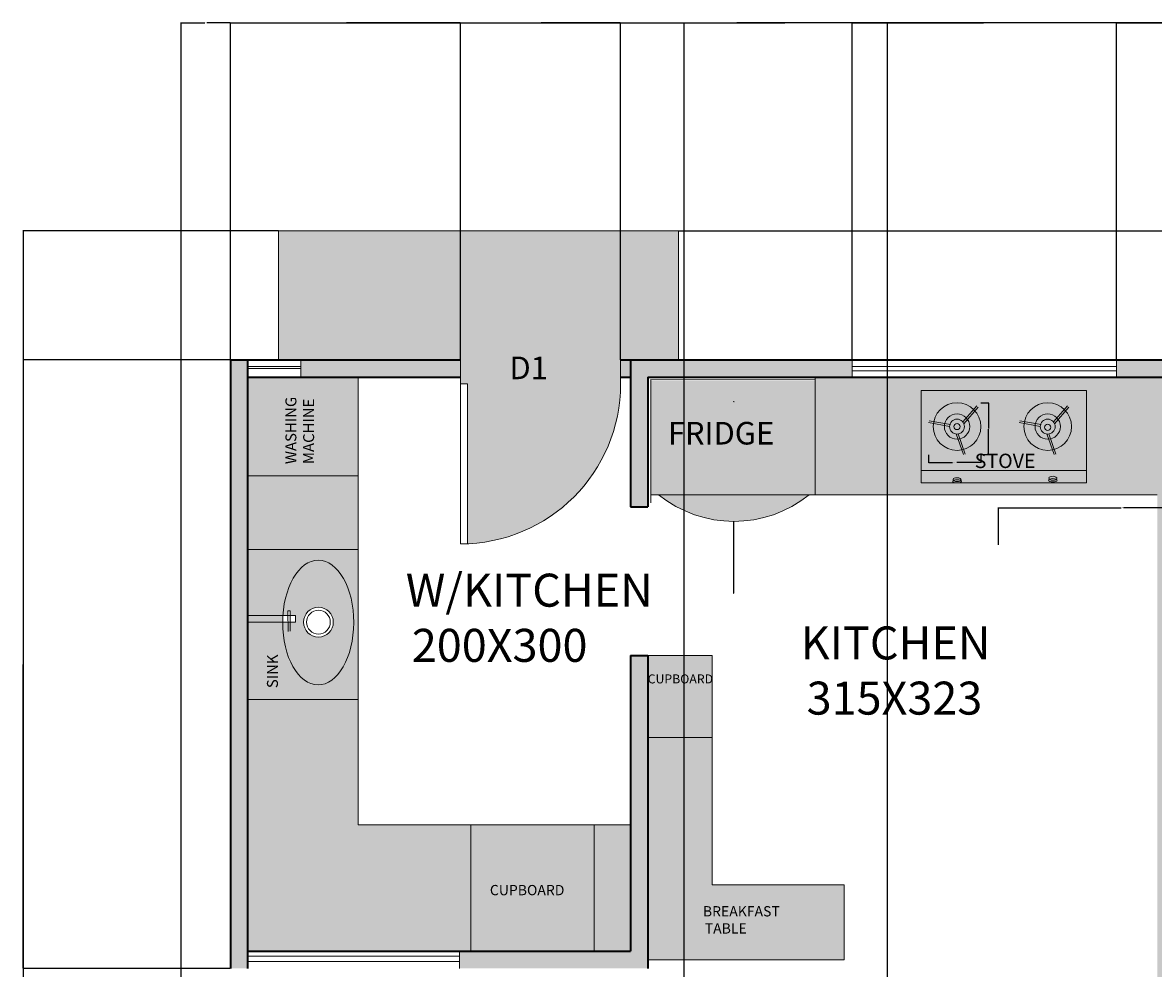
# Model space of a CAD drawing. Units: inches. Extents: x 192 to 1361, y -1362 to 367.
# Tile 19 of 23: x 192 to 783, y -127 to 367. Entities that reach past the tile are written whole.
import ezdxf

# ---------------------------------------------------------------- set-up
doc = ezdxf.new("R2010")
doc.units = ezdxf.units.IN
doc.header["$MEASUREMENT"] = 0
for name, color, linetype, lineweight in [('A-ANNO-DIMS', 2, 'Continuous', 18), ('A-AREA-IDEN', 7, 'Continuous', 18), ('A-DOOR', 4, 'Continuous', 18), ('A-EQPM', 8, 'Continuous', 18), ('A-FLOR-CASE', 32, 'Continuous', 18), ('A-FLOR-FIXT', 8, 'Continuous', 18), ('A-FLOR-STRS', 7, 'Continuous', 18), ('A-WALL-PATT', 250, 'Continuous', 13), ('text', 7, 'Continuous', 18), ('walls', 7, 'Continuous', 35), ('windows', 4, 'Continuous', 18)]:
    doc.layers.add(name, color=color, linetype=linetype, lineweight=lineweight)
for name, color, linetype, lineweight, true_color in [('A-EQPM-PATT', 251, 'Continuous', 13, 0x636466), ('A-FLOR-CASE-PATT', 9, 'Continuous', 13, 0xc7c8ca), ('A-FLOR-FIXT-PATT', 251, 'Continuous', 13, 0x636466), ('A-FLOR-STRS-PATT', 252, 'Continuous', 13, 0x939598)]:
    doc.layers.add(name, color=color, linetype=linetype, lineweight=lineweight, true_color=true_color)
doc.styles.get("Standard").update_dxf_attribs({"font": 'arial.ttf'})
doc.dimstyles.get("Standard").update_dxf_attribs({"dimtxt": 0.18, "dimasz": 0.18, "dimexe": 0.18, "dimexo": 0.0625, "dimgap": 0.09, "dimtad": 0, "dimtih": 1, "dimtoh": 1, "dimzin": 0, "dimdsep": 46, "dimlunit": 3, "dimtxsty": 'Standard', "dimcen": 0.09, "dimadec": 0, "dimazin": 0, "dimtfac": 1, "dimtofl": 0, "dimtmove": 0, "dimatfit": 3, "dimfxl": 1, "dimtolj": 1, "dimtzin": 0, "dimarcsym": 0})

# ---------------------------------------------------------------- blocks, each defined once
blk = doc.blocks.new('*U2')
for p, q in [((0, 0), (-1e-16, -5.999999999999999)), ((40, -6e-16), (40, -6))]:
    blk.add_line(p, q)
blk.add_lwpolyline([(0, 0), (5.6e-15, 40), (1.750000000000007, 40), (1.749999999999998, -7e-16)], close=True)
blk.add_arc((0, 0), 40, 0, 90)
blk = doc.blocks.new('COOKTOP-BURNER')
for p, q in [((2.998043829084622, 2.479431517935921), (10.32791550119827, 10.87990728422207)), ((3.605004346216333, 1.462802486064987), (11.02729633620413, 10.21636973317069)), ((-3.912598951481527, -2.84e-14), (-14.8525602053071, 2.147617193399554)), ((-3.335652644571382, 1.033957743843728), (-14.62761024594374, 3.085067534771468)), ((-0.5356780643953698, -3.853426587660607), (3.333987552905909, -14.65810362865281)), ((0.6482287596465995, -3.836097875688011), (4.258318341358403, -14.38419083685303))]:
    blk.add_line(p, q)
for radius in [12.42722873055866, 6.60613442143804, 3.890481648582393]:
    blk.add_circle((1.137e-13, -2.84e-14), radius)
blk = doc.blocks.new('*D37')
at = {"layer": 'A-ANNO-DIMS', "color": 0, "lineweight": -2, "transparency": 16777216}
for p, q in [((665.3194969474908, 141.5488445880535), (665.3194969474908, 137.3393762476736)), ((665.4994969474907, 137.5193762476736), (677.8694459856831, 137.5193762476736)), ((692.4192858833568, 137.5193762476736), (680.0493368451646, 137.5193762476736)), ((692.5992858833567, 141.5488445880535), (692.5992858833567, 137.3393762476736))]:
    blk.add_line(p, q, dxfattribs=at)
at = {"layer": 'A-ANNO-DIMS', "color": 0, "transparency": 16777216}
for points in [[(665.4994969474907, 137.5493762476736), (665.4994969474907, 137.4893762476736), (665.3194969474908, 137.5193762476736)], [(692.4192858833568, 137.5493762476736), (692.4192858833568, 137.4893762476736), (692.5992858833567, 137.5193762476736)]]:
    blk.add_solid(points, dxfattribs=at)
at = {"layer": 'Defpoints', "color": 0, "transparency": 16777216}
for p in [(665.3194969474908, 141.6113445880535), (692.5992858833567, 141.6113445880535), (692.5992858833567, 137.5193762476736)]:
    blk.add_point(p, dxfattribs=at)
at = {"layer": 'A-ANNO-DIMS', "color": 0, "transparency": 16777216, "insert": (678.9593914154239, 137.5193762476736), "char_height": 0.18, "attachment_point": 5}
blk.add_mtext('\\A1;BURNER 27 TYP.', dxfattribs=at)
blk = doc.blocks.new('*D38')
at = {"layer": 'A-ANNO-DIMS', "color": 0, "lineweight": -2, "transparency": 16777216}
for p, q in [((692.6617858833569, 168.696676947265), (696.871254223737, 168.696676947265)), ((696.6912542237371, 168.5166769472649), (696.6912542237371, 155.3344405084505)), ((696.6912542237371, 141.7913445880535), (696.6912542237371, 154.9735810268679)), ((692.6617858833569, 141.6113445880535), (696.871254223737, 141.6113445880535))]:
    blk.add_line(p, q, dxfattribs=at)
at = {"layer": 'A-ANNO-DIMS', "color": 0, "transparency": 16777216}
for points in [[(696.661254223737, 168.5166769472649), (696.7212542237371, 168.5166769472649), (696.6912542237371, 168.696676947265)], [(696.661254223737, 141.7913445880535), (696.7212542237371, 141.7913445880535), (696.6912542237371, 141.6113445880535)]]:
    blk.add_solid(points, dxfattribs=at)
at = {"layer": 'Defpoints', "color": 0, "transparency": 16777216}
for p in [(692.5992858833569, 168.696676947265), (696.6912542237371, 168.696676947265), (692.5992858833569, 141.6113445880535)]:
    blk.add_point(p, dxfattribs=at)
at = {"layer": 'A-ANNO-DIMS', "color": 0, "transparency": 16777216, "insert": (696.691254223737, 155.154010767659), "char_height": 0.18, "attachment_point": 5}
blk.add_mtext('\\A1;27 TYP.', dxfattribs=at)
blk = doc.blocks.new('*D45')
at = {"layer": 'A-ANNO-DIMS', "color": 0, "lineweight": -2, "transparency": 16777216}
for p, q in [((701.780963977869, 94.4585869856048), (701.780963977869, 113.9793046531113)), ((701.9609639778689, 113.7993046531113), (765.841371209712, 113.7993046531113)), ((830.9557484279125, 113.7993046531113), (767.0753411960693, 113.7993046531113)), ((831.1357484279124, 94.4585869856048), (831.1357484279124, 113.9793046531113))]:
    blk.add_line(p, q, dxfattribs=at)
at = {"layer": 'A-ANNO-DIMS', "color": 0, "transparency": 16777216}
for points in [[(701.9609639778689, 113.8293046531113), (701.9609639778689, 113.7693046531113), (701.780963977869, 113.7993046531113)], [(830.9557484279125, 113.8293046531113), (830.9557484279125, 113.7693046531113), (831.1357484279124, 113.7993046531113)]]:
    blk.add_solid(points, dxfattribs=at)
at = {"layer": 'Defpoints', "color": 0, "transparency": 16777216}
for p in [(701.780963977869, 113.7993046531113), (701.780963977869, 94.3960869856048), (831.1357484279124, 94.3960869856048)]:
    blk.add_point(p, dxfattribs=at)
at = {"layer": 'A-ANNO-DIMS', "color": 0, "transparency": 16777216, "insert": (766.4583562028906, 113.7993046531113), "char_height": 0.18, "attachment_point": 5}
blk.add_mtext('\\A1;SINK 129', dxfattribs=at)
blk = doc.blocks.new('*D48')
at = {"layer": 'A-ANNO-DIMS', "color": 0, "lineweight": -2, "transparency": 16777216}
for p, q in [((325.6332190000001, 258.5285980000001), (192.162545, 258.5285980000001)), ((192.3425450000001, 258.3485980000001), (192.3425450000002, -429.2150894706685)), ((192.3425450000004, -1117.142706), (192.3425450000002, -429.5790185293316)), ((395.2143240000002, -1117.322706), (192.1625450000004, -1117.322706))]:
    blk.add_line(p, q, dxfattribs=at)
at = {"layer": 'A-ANNO-DIMS', "color": 0, "transparency": 16777216}
for points in [[(192.312545, 258.3485980000001), (192.3725450000001, 258.3485980000001), (192.3425450000001, 258.5285980000001)], [(192.3125450000004, -1117.142706), (192.3725450000004, -1117.142706), (192.3425450000004, -1117.322706)]]:
    blk.add_solid(points, dxfattribs=at)
at = {"layer": 'Defpoints', "color": 0, "transparency": 16777216}
for p in [(325.6957190000001, 258.5285980000001), (192.3425450000004, -1117.322706), (395.2768240000002, -1117.322706)]:
    blk.add_point(p, dxfattribs=at)
at = {"layer": 'A-ANNO-DIMS', "color": 0, "transparency": 16777216, "insert": (192.342545, -429.397054), "char_height": 0.18, "attachment_point": 5}
blk.add_mtext('\\A1;1375.9', dxfattribs=at)
blk = doc.blocks.new('*D49')
at = {"layer": 'A-ANNO-DIMS', "color": 0, "lineweight": -2, "transparency": 16777216}
for p, q in [((274.892545, -399.349572), (274.8925450000001, 367.389667)), ((275.072545, 367.209667), (287.2537032892224, 367.209667)), ((300.365189, 367.209667), (288.1840307107777, 367.209667)), ((300.545189, 191.164493), (300.545189, 367.389667))]:
    blk.add_line(p, q, dxfattribs=at)
at = {"layer": 'A-ANNO-DIMS', "color": 0, "transparency": 16777216}
for points in [[(275.072545, 367.239667), (275.072545, 367.179667), (274.8925450000001, 367.209667)], [(300.365189, 367.239667), (300.365189, 367.179667), (300.545189, 367.209667)]]:
    blk.add_solid(points, dxfattribs=at)
at = {"layer": 'Defpoints', "color": 0, "transparency": 16777216}
for p in [(300.545189, 367.209667), (300.545189, 191.101993), (274.892545, -399.412072)]:
    blk.add_point(p, dxfattribs=at)
at = {"layer": 'A-ANNO-DIMS', "color": 0, "transparency": 16777216, "insert": (287.7188670000001, 367.209667), "char_height": 0.18, "attachment_point": 5}
blk.add_mtext('\\A1;25.653', dxfattribs=at)
blk = doc.blocks.new('*D50')
at = {"layer": 'A-ANNO-DIMS', "color": 0, "lineweight": -2, "transparency": 16777216}
for p, q in [((300.545189, 191.164493), (300.545189, 367.389667)), ((300.725189, 367.209667), (571.3556178929057, 367.209667)), ((842.772718, 367.209667), (572.1422891070941, 367.209667)), ((842.952718, 192.111569), (842.952718, 367.389667))]:
    blk.add_line(p, q, dxfattribs=at)
at = {"layer": 'A-ANNO-DIMS', "color": 0, "transparency": 16777216}
for points in [[(300.725189, 367.239667), (300.725189, 367.179667), (300.545189, 367.209667)], [(842.772718, 367.239667), (842.772718, 367.179667), (842.952718, 367.209667)]]:
    blk.add_solid(points, dxfattribs=at)
at = {"layer": 'Defpoints', "color": 0, "transparency": 16777216}
for p in [(842.952718, 367.209667), (300.545189, 191.101993), (842.952718, 192.049069)]:
    blk.add_point(p, dxfattribs=at)
at = {"layer": 'A-ANNO-DIMS', "color": 0, "transparency": 16777216, "insert": (571.7489534999999, 367.209667), "char_height": 0.18, "attachment_point": 5}
blk.add_mtext('\\A1;542.4', dxfattribs=at)
blk = doc.blocks.new('*D53')
at = {"layer": 'A-ANNO-DIMS', "color": 0, "lineweight": -2, "transparency": 16777216}
for p, q in [((534.6874480000002, 258.5285980000001), (1360.413144000001, 258.5285980000002)), ((1360.233144000001, 258.3485980000002), (1360.233144000001, 225.4707366377901)), ((1360.233144000001, 192.2290690000002), (1360.233144000001, 225.1069303622103)), ((843.0152180000003, 192.0490690000001), (1360.413144000001, 192.0490690000002))]:
    blk.add_line(p, q, dxfattribs=at)
at = {"layer": 'A-ANNO-DIMS', "color": 0, "transparency": 16777216}
for points in [[(1360.203144000001, 258.3485980000002), (1360.263144000001, 258.3485980000002), (1360.233144000001, 258.5285980000002)], [(1360.203144000001, 192.2290690000002), (1360.263144000001, 192.2290690000002), (1360.233144000001, 192.0490690000002)]]:
    blk.add_solid(points, dxfattribs=at)
at = {"layer": 'Defpoints', "color": 0, "transparency": 16777216}
for p in [(534.6249480000002, 258.5285980000001), (1360.233144000001, 258.5285980000002), (842.9527180000003, 192.0490690000001)]:
    blk.add_point(p, dxfattribs=at)
at = {"layer": 'A-ANNO-DIMS', "color": 0, "transparency": 16777216, "insert": (1360.233144000001, 225.2888334999997), "char_height": 0.18, "attachment_point": 5}
blk.add_mtext('\\A1;66.48', dxfattribs=at)
blk = doc.blocks.new('*D61')
at = {"layer": 'A-ANNO-DIMS', "color": 0, "lineweight": -2, "transparency": 16777216}
for p, q in [((300.545189, 191.164493), (300.545189, 367.389667)), ((300.725189, 367.209667), (360.215756803547, 367.209667)), ((420.6179889999999, 367.209667), (361.1274211964529, 367.209667)), ((420.7979889999999, 191.164493), (420.7979889999999, 367.389667))]:
    blk.add_line(p, q, dxfattribs=at)
at = {"layer": 'A-ANNO-DIMS', "color": 0, "transparency": 16777216}
for points in [[(300.725189, 367.239667), (300.725189, 367.179667), (300.545189, 367.209667)], [(420.6179889999999, 367.239667), (420.6179889999999, 367.179667), (420.7979889999999, 367.209667)]]:
    blk.add_solid(points, dxfattribs=at)
at = {"layer": 'Defpoints', "color": 0, "transparency": 16777216}
for p in [(420.7979889999999, 367.209667), (300.545189, 191.101993), (420.7979889999999, 191.101993)]:
    blk.add_point(p, dxfattribs=at)
at = {"layer": 'A-ANNO-DIMS', "color": 0, "transparency": 16777216, "insert": (360.671589, 367.209667), "char_height": 0.18, "attachment_point": 5}
blk.add_mtext('\\A1;120.25', dxfattribs=at)
blk = doc.blocks.new('*D62')
at = {"layer": 'A-ANNO-DIMS', "color": 0, "lineweight": -2, "transparency": 16777216}
for p, q in [((420.7979889999999, 191.164493), (420.7979889999999, 367.389667)), ((420.977989, 367.209667), (462.2743081180082, 367.209667)), ((504.218308, 367.209667), (462.9219888819918, 367.209667)), ((504.398308, 191.164493), (504.398308, 367.389667))]:
    blk.add_line(p, q, dxfattribs=at)
at = {"layer": 'A-ANNO-DIMS', "color": 0, "transparency": 16777216}
for points in [[(420.977989, 367.239667), (420.977989, 367.179667), (420.7979889999999, 367.209667)], [(504.218308, 367.239667), (504.218308, 367.179667), (504.398308, 367.209667)]]:
    blk.add_solid(points, dxfattribs=at)
at = {"layer": 'Defpoints', "color": 0, "transparency": 16777216}
for p in [(504.398308, 367.209667), (420.7979889999999, 191.101993), (504.398308, 191.101993)]:
    blk.add_point(p, dxfattribs=at)
at = {"layer": 'A-ANNO-DIMS', "color": 0, "transparency": 16777216, "insert": (462.5981484999999, 367.209667), "char_height": 0.18, "attachment_point": 5}
blk.add_mtext('\\A1;83.6', dxfattribs=at)
blk = doc.blocks.new('*D63')
at = {"layer": 'A-ANNO-DIMS', "color": 0, "lineweight": -2, "transparency": 16777216}
for p, q in [((504.398308, 191.164493), (504.398308, 367.389667)), ((504.5783079999999, 367.209667), (564.6372506357435, 367.209667)), ((625.222196, 367.209667), (565.1632533642565, 367.209667)), ((625.402196, 191.164493), (625.402196, 367.389667))]:
    blk.add_line(p, q, dxfattribs=at)
at = {"layer": 'A-ANNO-DIMS', "color": 0, "transparency": 16777216}
for points in [[(504.5783079999999, 367.239667), (504.5783079999999, 367.179667), (504.398308, 367.209667)], [(625.222196, 367.239667), (625.222196, 367.179667), (625.402196, 367.209667)]]:
    blk.add_solid(points, dxfattribs=at)
at = {"layer": 'Defpoints', "color": 0, "transparency": 16777216}
for p in [(625.402196, 367.209667), (504.398308, 191.101993), (625.402196, 191.101993)]:
    blk.add_point(p, dxfattribs=at)
at = {"layer": 'A-ANNO-DIMS', "color": 0, "transparency": 16777216, "insert": (564.900252, 367.209667), "char_height": 0.18, "attachment_point": 5}
blk.add_mtext('\\A1;121', dxfattribs=at)
blk = doc.blocks.new('*D64')
at = {"layer": 'A-ANNO-DIMS', "color": 0, "lineweight": -2, "transparency": 16777216}
for p, q in [((625.402196, 191.164493), (625.402196, 367.389667)), ((625.582196, 367.209667), (693.9681959597544, 367.209667)), ((763.2637729999999, 367.209667), (694.8777730402455, 367.209667)), ((763.443773, 191.164493), (763.443773, 367.389667))]:
    blk.add_line(p, q, dxfattribs=at)
at = {"layer": 'A-ANNO-DIMS', "color": 0, "transparency": 16777216}
for points in [[(625.582196, 367.239667), (625.582196, 367.179667), (625.402196, 367.209667)], [(763.2637729999999, 367.239667), (763.2637729999999, 367.179667), (763.443773, 367.209667)]]:
    blk.add_solid(points, dxfattribs=at)
at = {"layer": 'Defpoints', "color": 0, "transparency": 16777216}
for p in [(763.443773, 367.209667), (625.402196, 191.101993), (763.443773, 191.101993)]:
    blk.add_point(p, dxfattribs=at)
at = {"layer": 'A-ANNO-DIMS', "color": 0, "transparency": 16777216, "insert": (694.4229844999999, 367.209667), "char_height": 0.18, "attachment_point": 5}
blk.add_mtext('\\A1;138.04', dxfattribs=at)
blk = doc.blocks.new('*D65')
at = {"layer": 'A-ANNO-DIMS', "color": 0, "lineweight": -2, "transparency": 16777216}
for p, q in [((763.443773, 191.164493), (763.443773, 367.389667)), ((763.6237729999999, 367.209667), (802.6888125143246, 367.209667)), ((842.365189, 367.209667), (803.3001494856751, 367.209667)), ((842.545189, 191.164493), (842.545189, 367.389667))]:
    blk.add_line(p, q, dxfattribs=at)
at = {"layer": 'A-ANNO-DIMS', "color": 0, "transparency": 16777216}
for points in [[(763.6237729999999, 367.239667), (763.6237729999999, 367.179667), (763.443773, 367.209667)], [(842.365189, 367.239667), (842.365189, 367.179667), (842.545189, 367.209667)]]:
    blk.add_solid(points, dxfattribs=at)
at = {"layer": 'Defpoints', "color": 0, "transparency": 16777216}
for p in [(842.545189, 367.209667), (763.443773, 191.101993), (842.545189, 191.101993)]:
    blk.add_point(p, dxfattribs=at)
at = {"layer": 'A-ANNO-DIMS', "color": 0, "transparency": 16777216, "insert": (802.994481, 367.209667), "char_height": 0.18, "attachment_point": 5}
blk.add_mtext('\\A1;79.1', dxfattribs=at)
blk = doc.blocks.new('*D66')
at = {"layer": 'A-ANNO-DIMS', "color": 0, "lineweight": -2, "transparency": 16777216}
for p, q in [((300.4826890000001, 191.101993), (192.1625450000002, 191.101993)), ((192.3425450000002, 190.921993), (192.3425450000002, 32.28395752933149)), ((192.3425450000002, -126.7180070000001), (192.3425450000002, 31.92002847066847)), ((300.4826890000001, -126.898007), (192.1625450000002, -126.8980070000001))]:
    blk.add_line(p, q, dxfattribs=at)
at = {"layer": 'A-ANNO-DIMS', "color": 0, "transparency": 16777216}
for points in [[(192.3125450000002, 190.921993), (192.3725450000002, 190.921993), (192.3425450000002, 191.101993)], [(192.3125450000002, -126.7180070000001), (192.3725450000002, -126.7180070000001), (192.3425450000002, -126.8980070000001)]]:
    blk.add_solid(points, dxfattribs=at)
at = {"layer": 'Defpoints', "color": 0, "transparency": 16777216}
for p in [(300.5451890000001, 191.101993), (192.3425450000002, -126.8980070000001), (300.5451890000001, -126.898007)]:
    blk.add_point(p, dxfattribs=at)
at = {"layer": 'A-ANNO-DIMS', "color": 0, "transparency": 16777216, "insert": (192.3425450000002, 32.10199299999992), "char_height": 0.18, "attachment_point": 5}
blk.add_mtext('\\A1;318', dxfattribs=at)
blk = doc.blocks.new('*D70')
at = {"layer": 'A-ANNO-DIMS', "color": 0, "lineweight": -2, "transparency": 16777216}
for p, q in [((537.571706, -441.835507), (537.571706, 367.389667)), ((537.7517059999998, 367.209667), (590.2778894836289, 367.209667)), ((643.712545, 367.209667), (591.1863615163709, 367.209667)), ((643.892545, -441.835507), (643.892545, 367.389667))]:
    blk.add_line(p, q, dxfattribs=at)
at = {"layer": 'A-ANNO-DIMS', "color": 0, "transparency": 16777216}
for points in [[(537.7517059999998, 367.239667), (537.7517059999998, 367.179667), (537.571706, 367.209667)], [(643.712545, 367.239667), (643.712545, 367.179667), (643.892545, 367.209667)]]:
    blk.add_solid(points, dxfattribs=at)
at = {"layer": 'Defpoints', "color": 0, "transparency": 16777216}
for p in [(643.892545, 367.209667), (537.571706, -441.8980069999999), (643.892545, -441.8980069999999)]:
    blk.add_point(p, dxfattribs=at)
at = {"layer": 'A-ANNO-DIMS', "color": 0, "transparency": 16777216, "insert": (590.7321254999999, 367.209667), "char_height": 0.18, "attachment_point": 5}
blk.add_mtext('\\A1;106.32', dxfattribs=at)
blk = doc.blocks.new('*D73')
at = {"layer": 'A-ANNO-DIMS', "color": 0, "lineweight": -2, "transparency": 16777216}
for p, q in [((563.5042099999997, 169.3224309999999), (563.6842099999996, 169.3224309999999)), ((563.5942099999996, 169.2324309999999), (563.5942099999996, 169.4124309999999)), ((563.5938739999978, 69.15581280021131), (563.5939993962058, 106.538295000001)), ((563.4138739999979, 69.1558128002113), (563.5938739999978, 69.15581280021131))]:
    blk.add_line(p, q, dxfattribs=at)
at = {"layer": 'A-ANNO-DIMS', "color": 0, "transparency": 16777216}
blk.add_solid([(563.5639993962061, 106.5382951006333), (563.6239993962057, 106.5382948993686), (563.5939999999997, 106.7182949999999)], dxfattribs=at)
at = {"layer": 'Defpoints', "color": 0, "transparency": 16777216}
for p in [(563.5942099999997, 169.3224309999999), (563.5939999999997, 106.7182949999999)]:
    blk.add_point(p, dxfattribs=at)
at = {"layer": 'A-ANNO-DIMS', "color": 0, "transparency": 16777216, "insert": (563.0040240682107, 69.15581280021142), "char_height": 0.18, "attachment_point": 5}
blk.add_mtext('\\A1;R62.6', dxfattribs=at)

msp = doc.modelspace()

# ---------------------------------------------------------------- hatches: boundary and pattern name
at = {"layer": 'A-EQPM-PATT'}
h = msp.add_hatch(color=256, dxfattribs=at)
h.dxf.hatch_style = 1
h.paths.add_polyline_path([(520.1272786621957, 180.37523831581), (520.1272786621957, 120.6542820654139), (606.0055655280232, 120.6542820654139), (606.0055655280232, 180.37523831581)])
h.paths.add_polyline_path([(524.2154194657116, 120.6542820654139, 0.3538957662438658), (602.9730012785246, 120.6542820654139)])
h = msp.add_hatch(color=256, dxfattribs=at)
h.dxf.hatch_style = 1
h.paths.add_polyline_path([(654.6941349520653, 133.2965860047039, 0.4472035247863919), (664.4676486712701, 125.6924393581307), (747.8111784828459, 125.6924393581307, 0.3244181347622925), (755.5844684036286, 130.1594570450853), (755.5844684036286, 176.3328940198642, 0.3295456964687013), (747.8111785084185, 181.0248198872323), (661.4957202282897, 181.0248198853133, 0.2614299454499895), (654.6941349520653, 176.569079923764)])
h.paths.add_polyline_path([(667.7448284222395, 156.2694482167063, -1), (692.5992858833569, 156.2694482167063, -1)], flags=16)
h.paths.add_polyline_path([(673.56592273136, 156.2694482167063, -1), (686.778191574236, 156.2694482167063, -1)], flags=0)
h.paths.add_polyline_path([(676.2815755042159, 156.2694482167063, -1), (684.0625388013804, 156.2694482167063, -1)], flags=0)
edge = h.paths.add_edge_path(flags=16)
edge.add_ellipse((680.1596553194548, 127.6653223792632), major_axis=(-2.265511773118937, 0.0641621067748367), ratio=0.3769733725084229, start_angle=41.86570148013669, end_angle=148.3082686719917, ccw=False)
edge.add_ellipse((680.1596553194548, 127.6653223792632), major_axis=(-2.265511773118937, 0.0641621067748367), ratio=0.3769733725084229, start_angle=346.4338229157989, end_angle=401.8657014801367, ccw=False)
edge.add_ellipse((680.1838427235941, 128.5193599934903), major_axis=(-2.108826373640958, 0.136184926067124), ratio=0.4928397098496223, start_angle=169.7196154411588, end_angle=373.72857998463945, ccw=False)
edge.add_ellipse((680.1596553194548, 127.6653223792632), major_axis=(-2.265511773118937, 0.0641621067748367), ratio=0.3769733725084229, start_angle=148.3082686719917, end_angle=192.1304824464878, ccw=False)
h.paths.add_polyline_path([(715.1179190683129, 156.2694482167063, -1), (739.9723765294304, 156.2694482167063, -1)], flags=16)
h.paths.add_polyline_path([(734.1512822203096, 156.2694482167063, -1), (720.9390133774338, 156.2694482167063, -1)], flags=0)
h.paths.add_polyline_path([(731.4356294474538, 156.2694482167063, -1), (723.6546661502894, 156.2694482167063, -1)], flags=0)
h.paths.add_polyline_path([(678.5618801005874, 156.2694482167063, -1), (681.7822342050089, 156.2694482167063, -1)], flags=0)
h.paths.add_polyline_path([(725.934970746661, 156.2694482167063, -1), (729.1553248510824, 156.2694482167063, -1)], flags=0)
edge = h.paths.add_edge_path(flags=16)
edge.add_ellipse((730.2790187730303, 129.2411328864045), major_axis=(-2.108826373640957, 0.1361849260671237), ratio=0.4928397098496223, start_angle=165.0804609789027, end_angle=377.6699463424078, ccw=False)
edge.add_ellipse((730.2119014335817, 128.2018195082961), major_axis=(-2.265511773118937, 0.0641621067748368), ratio=0.3769733725084229, start_angle=342.9101370313131, end_angle=554.300550688774, ccw=False)
at = {"layer": 'A-FLOR-CASE-PATT'}
h = msp.add_hatch(color=256, dxfattribs=at)
h.dxf.hatch_style = 1
h.paths.add_polyline_path([(367.2563921661531, 182.101992675173), (309.5451889353615, 182.101992675173), (309.5451889353615, 130.5475761196903), (367.2563921661531, 130.5475761196903)])
h.paths.add_polyline_path([(367.2563921661531, 13.5566443611624), (309.5451889353615, 13.55664436116237), (309.5451889353615, -117.8980073248269), (426.1374151077765, -117.8980073248269), (426.1374151077765, -51.88342877959076), (367.2563921661531, -51.88342877959076)])
h.paths.add_polyline_path([(367.2563921661531, 130.5475761196903), (309.5451889353615, 130.5475761196903), (309.5451889353615, 91.98957794753846), (367.2563921661531, 91.98957794753848)])
h.paths.add_polyline_path([(490.5683664073912, -51.88342877959076), (426.1374151077765, -51.88342877959079), (426.1374151077765, -117.8980073248269), (490.5683664073913, -117.8980073248269)])
h.paths.add_polyline_path([(509.5451889353614, -51.88342877959076), (490.5683664073912, -51.88342877959076), (490.5683664073913, -117.8980073248269), (509.5451889353614, -117.8980073248269)])
h.paths.add_polyline_path([(552.3161055696219, -6.213326217646681), (518.5451889353614, -6.213326217646681), (518.5451889353614, -122.3395355970042), (621.252934446602, -122.3395355970042), (621.252934446602, -83.2276039636199), (552.3161055696219, -83.22760396361988)])
h.paths.add_polyline_path([(552.3161055696219, 36.60199267517304), (518.5451889353614, 36.60199267517304), (518.5451889353614, -6.213326217646681), (552.3161055696219, -6.213326217646653)])
h = msp.add_hatch(color=256, dxfattribs=at)
h.dxf.hatch_style = 1
h.paths.add_polyline_path([(833.5451889353615, 182.101992675173), (606.035314480534, 182.101992675173), (606.0320695517825, 180.6287964589344), (606.109309992806, 180.6286263256385), (606.0055655280232, 120.6542820654139), (784.8041419739257, 120.6542820658329), (784.8041419739257, -60.49958728474123), (833.5451889353615, -60.49958728474118)])
at = {"layer": 'A-FLOR-FIXT-PATT'}
h = msp.add_hatch(color=256, dxfattribs=at)
h.dxf.hatch_style = 1
edge = h.paths.add_edge_path()
edge.add_ellipse((346.4015860498506, 53.86014095233496), major_axis=(0.0897725345072745, 32.61993048690351), ratio=0.568990406928987, start_angle=89.77278696833508, end_angle=78.68100194365468, ccw=False)
edge.add_line((327.8414083400814, 53.98482425088332), (309.5451889353615, 53.98482425088332))
edge.add_line((309.5451889353615, 53.98482425088332), (309.5451889353615, 13.5566443611624))
edge.add_line((309.5451889353615, 13.5566443611624), (367.2563921661531, 13.5566443611624))
edge.add_line((367.2563921661531, 13.5566443611624), (367.2563921661531, 91.98957794753846))
edge.add_line((367.2563921661531, 91.98957794753848), (309.5451889353615, 91.98957794753846))
edge.add_line((309.5451889353615, 91.98957794753846), (309.5451889353615, 57.60216911136854))
edge.add_line((309.5451889353615, 57.60216911136854), (327.9705352807811, 57.60216911136854))
edge = h.paths.add_edge_path(flags=17)
edge.add_ellipse((346.4015860498506, 53.86014095233496), major_axis=(0.0897725345072745, 32.61993048690351), ratio=0.568990406928987, start_angle=-270.227213031665, end_angle=78.68100194365473)
edge.add_line((327.9705352807811, 57.60216911136854), (330.5969786775669, 57.60216911136854))
edge.add_line((330.5969786775669, 57.60216911136854), (330.5859614346086, 59.90799801485451))
edge.add_line((330.5859614346086, 59.90799801485451), (331.7591235928912, 59.91360337980977))
edge.add_line((331.7591235928912, 59.91360337980977), (331.7701676182649, 57.60216911136854))
edge.add_line((331.7701676182649, 57.60216911136854), (334.4929653930154, 57.60216911136854))
edge.add_line((334.4929653930154, 57.60216911136854), (334.5102490549264, 53.98482425088332))
edge.add_line((334.5102490549264, 53.98482425088332), (327.8414083400814, 53.98482425088332))
h.paths.add_polyline_path([(338.7613475983098, 54.04226685662357, -1), (354.3037905554878, 54.04226685662357, -1)], flags=16)
h.paths.add_polyline_path([(340.3275509583993, 54.04226685662357, -1), (352.7375871953983, 54.04226685662357, -1)], flags=0)
h.paths.add_polyline_path([(352.7375871953983, 54.04226685662357, 1), (340.3275509583993, 54.04226685662357, 1)], flags=0)
edge = h.paths.add_edge_path(flags=17)
edge.add_ellipse((346.4015860498506, 53.86014095233496), major_axis=(0.0897725345072745, 32.61993048690351), ratio=0.568990406928987, start_angle=78.68100194365468, end_angle=89.77278696833503, ccw=False)
edge.add_line((327.9705352807811, 57.60216911136854), (309.5451889353615, 57.60216911136854))
edge.add_line((309.5451889353615, 57.60216911136854), (309.5451889353615, 53.98482425088332))
edge.add_line((309.5451889353615, 53.98482425088332), (327.8414083400814, 53.98482425088332))
at = {"layer": 'A-FLOR-STRS-PATT'}
h = msp.add_hatch(color=256, dxfattribs=at)
h.dxf.hatch_style = 1
h.paths.add_polyline_path([(534.6249481233752, 258.5285978964557), (325.6957187905937, 258.5285978964557), (325.6957187905937, 191.101992675173), (420.7979888647932, 191.101992675173), (420.7979888647932, 178.5619448757428), (424.4555028062937, 178.5619448757428), (424.4555028062937, 95.0416726521634, 0.4014527144963572), (504.3983075276613, 178.5619448757428), (504.3983075276613, 191.101992675173), (534.6249481233752, 191.101992675173)])
at = {"layer": 'A-WALL-PATT'}
h = msp.add_hatch(color=256, dxfattribs=at)
h.dxf.hatch_style = 1
h.paths.add_polyline_path([(309.5451889353615, 191.101992675173), (300.5451889353615, 191.101992675173), (300.5451889353615, -126.898007324827), (309.5451889353615, -126.8980073248269), (309.5451889353615, -117.8980073248269)])
h.paths.add_polyline_path([(420.7979888647932, 191.101992675173), (337.3228677063344, 191.101992675173), (337.3228677063344, 182.101992675173), (420.7979888647932, 182.101992675173)])
h.paths.add_polyline_path([(518.5451889353614, 182.101992675173), (625.402196435898, 182.101992675173), (625.402196435898, 191.101992675173), (509.5451889353614, 191.101992675173), (509.5451889353614, 114.3261562634452), (518.5451889353614, 114.3261562634452)])
h.paths.add_polyline_path([(842.5451889353615, 191.101992675173), (763.4437725118987, 191.101992675173), (763.4437725118989, 182.101992675173), (833.5451889353615, 182.101992675173), (833.5451889353614, 161.1615418579658), (836.8088208065492, 161.1615418579658), (842.5451889353615, 161.1615418579658)])
h.paths.add_polyline_path([(842.5451889353615, -16.5674928553999), (833.5451889353614, -16.56749285539987), (833.5451889353614, -60.49958728474121), (784.8041419739257, -60.49958728474123), (784.8041419739257, -354.6796217638267), (793.8041419739257, -354.6796217638266), (793.8041419739257, -69.49958728474121), (1094.125155398258, -69.49958728474121), (1094.125155398258, -60.49958728474121), (842.5451889353615, -60.49958728474121)])
h.paths.add_polyline_path([(518.5451889353614, 36.60199267517305), (509.5451889353614, 36.60199267517304), (509.5451889353614, -117.8980073248269), (420.2204344382116, -117.8980073248269), (420.2204344382116, -126.898007324827), (518.5451889353614, -126.898007324827)])
h.paths.add_polyline_path([(474.8041419739258, -377.0384258897093), (465.8041419739257, -377.0384258897092), (465.8041419739257, -381.5384258897093), (465.8041419739257, -450.8980073248269), (537.5717061213309, -450.8980073248269), (537.5717061213307, -441.8980073248268), (474.8041419739258, -441.8980073248268)])
h.paths.add_polyline_path([(1162.804141973925, -380.6762896854179), (1204.300070955153, -380.676289685418), (1204.300070955153, -375.6762896854179), (1195.147073967669, -375.6762896854179), (1153.804141973926, -375.6762896854179), (1153.804141973926, -448.4995872847412), (856.5690753709177, -448.4995872847412), (856.5690753709177, -457.499587284741), (1162.804141973925, -457.4995872847412)])
h.paths.add_polyline_path([(1162.804141973925, -525.128007319321), (1153.804141973926, -525.128007319321), (1153.804141973926, -597.4995872847411), (1162.804141973925, -597.4995872847408)], flags=17)
h.paths.add_polyline_path([(1162.804141973925, -60.49958728474121), (1153.804141973926, -60.49958728474121), (1153.804141973926, -69.49958728474121), (1153.804141973926, -177.4732950264469), (1205.888928875302, -177.4732950264469), (1205.888928875302, -172.4732950264469), (1162.804141973925, -172.473295026447)])
h.paths.add_polyline_path([(980.5798651633768, -525.6860130712009), (971.5798651633768, -525.6860130712007), (971.5798651633768, -597.4995872847411), (980.5798651633768, -597.4995872847411)], flags=17)
h.paths.add_polyline_path([(856.5690753709177, -448.4995872847413), (798.7541670773728, -448.4995872847413), (784.8041419739257, -448.4995872847413), (784.8041419739257, -457.4995872847413), (847.5690753709177, -457.4995872847412), (847.5690753709177, -597.4995872847411), (784.8041419739257, -597.4995872847411), (784.8041419739257, -606.4995872847411), (1273.565765398564, -606.4995872847411), (1273.565765398564, -597.4995872847411), (856.5690753709177, -597.4995872847411)])
h.paths.add_polyline_path([(1273.565765398564, -773.8919522895034), (1099.836601134898, -773.8919522895034), (1099.836601134898, -851.9361992714873), (1108.836601134898, -851.9361992714873), (1108.836601134898, -782.8919522895034), (1273.565765398564, -782.8919522895034)])
h.paths.add_polyline_path([(1108.836601134898, -982.9213770098904), (1099.836601134898, -982.9213770098906), (1099.836601134898, -1067.624587332624), (1037.756291549154, -1067.624587332624), (1037.756291549154, -1076.624587332624), (1108.836601134898, -1076.624587332624)])
h.paths.add_polyline_path([(835.0779955891157, -1067.624587332624), (758.8457689766901, -1067.624587332624), (758.8457689766902, -940.2324367059535), (749.8457689766901, -940.2324367059538), (749.8457689766901, -963.1720045953997), (749.8457689766901, -970.4644011765903), (749.8457689766901, -1076.624587332624), (835.0779955891157, -1076.624587332624)])
h.paths.add_polyline_path([(450.3070229383964, -1066.98378940351), (441.3070229383965, -1066.98378940351), (441.3070229383965, -1076.624587332624), (450.3070229383965, -1076.624587332624)])
h.paths.add_polyline_path([(492.8925450663919, -756.4414928502347), (274.8925450663919, -756.4414928502347), (274.8925450663919, -765.4414928502347), (492.8925450663919, -765.4414928502347)])
h.paths.add_polyline_path([(283.8925450663919, -835.2244016542135), (274.8925450663919, -835.2244016542135), (274.8925450663919, -914.4414928502346), (492.8925450663919, -914.4414928502346), (492.8925450663919, -839.9414928502348), (483.8925450663918, -839.9414928502345), (483.8925450663918, -905.4414928502346), (283.8925450663919, -905.4414928502346)])
h.paths.add_polyline_path([(283.8925450663919, -441.898007324827), (283.8925450663918, -375.4296017141059), (281.6021282613037, -375.429601714106), (281.6021282613036, -399.4120715247955), (274.8925450663919, -399.4120715247954), (274.8925450663919, -441.898007324827), (274.8925450663919, -684.5088577166042), (283.8925450663919, -684.5088577166042)])
h = msp.add_hatch(color=256, dxfattribs=at)
h.dxf.hatch_style = 1
h.paths.add_polyline_path([(652.8925450663919, -441.898007324827), (643.8925450663918, -441.898007324827), (643.8925450663918, -457.846133166586), (643.8925450663918, -564.1669721116469), (643.8925450663918, -905.4414928502346), (578.0244629257031, -905.4414928502346), (578.0244629257031, -914.4414928502346), (643.8925450663918, -914.4414928502346), (643.8925450663918, -969.5483657063114), (652.6138145608154, -969.5483657063114), (652.6138145608154, -963.1720045953997), (652.6138145608154, -914.5560273874624)])
h.paths.add_polyline_path([(509.5451889353614, 191.101992675173), (504.3983075276613, 191.1019926751729), (504.3983075276613, 182.1019926751729), (509.5451889353614, 182.1019926751731)])

# ---------------------------------------------------------------- linework, layer by layer
at = {"layer": 'A-EQPM'}
for p, q in [((520.1272786621957, 120.6542820654139), (520.1272786621957, 180.8180142445744)), ((520.1272786621957, 180.8180142445744), (606.109309992806, 180.6286263256385)), ((606.109309992806, 180.6286263256385), (606.0055655280232, 120.6542820654139)), ((661.4957202312175, 175.0385616355948), (661.4957202312175, 126.9029761155034)), ((747.8111785069199, 175.0385616355948), (661.4957202312175, 175.0385616355948)), ((747.8111785069195, 126.9029761155034), (747.8111785069199, 175.0385616355948)), ((520.1272786621957, 116.3888405289696), (520.1272786621957, 161.1454192932534)), ((661.4957202312175, 133.2965860174828), (747.8111785069199, 133.2965860174828)), ((747.8111785069195, 126.9029761155034), (661.4957202312175, 126.9029761155034)), ((606.0055655280232, 120.6542820654139), (520.1272786621957, 120.6542820654139)), ((606.0055655280232, 120.6542820654139), (602.9730012785151, 120.6542820654068))]:
    msp.add_line(p, q, dxfattribs=at)
for centre in [(680.1720571527981, 156.2694482167063), (727.5595086581566, 155.904968577457)]:
    msp.add_circle(centre, 1.610177052210564, dxfattribs=at)
msp.add_arc((563.5942103721195, 169.3224313615276), 62.60413667769229, 231.0226883866979, 308.9773116133019, dxfattribs=at)
for centre, major_axis, ratio in [((730.2790187730303, 129.2411328864045), (-2.108826373640957, 0.1361849260671237), 0.4928397098496223), ((680.1596553194548, 127.6653223792632), (-2.265511773118937, 0.0641621067748367), 0.3769733725084229), ((680.1838427235941, 128.5193599934903), (-2.108826373640957, 0.1361849260671239), 0.4928397098496223), ((730.2119014335817, 128.2018195082961), (-2.265511773118937, 0.0641621067748368), 0.3769733725084229)]:
    msp.add_ellipse(centre, major_axis=major_axis, ratio=ratio, dxfattribs=at)
at = {"layer": 'A-FLOR-CASE'}
for p, q in [((367.2563921661531, 182.101992675173), (367.2563921661531, -51.88342877959076)), ((606.035314480534, 182.101992675173), (606.0320695517825, 180.6287964589344)), ((309.5451889353615, 130.5475761196903), (367.2563921661531, 130.5475761196903)), ((784.8041419739257, 120.6542820658329), (606.0055655280232, 120.6542820654139)), ((309.5451889353615, 91.98957794753846), (367.2563921661531, 91.98957794753848)), ((552.3161055696219, 36.60199267517305), (518.5451889353614, 36.60199267517305)), ((552.3161055696219, -83.2276039636199), (552.3161055696219, 36.60199267517305)), ((309.5451889353615, 13.5566443611624), (367.2563921661531, 13.5566443611624)), ((518.5451889353614, -6.213326217646681), (552.3161055696219, -6.213326217646681)), ((367.2563921661531, -51.88342877959076), (509.5451889353614, -51.88342877959076)), ((426.1374151077765, -51.88342877959076), (426.1374151077765, -117.8980073248269)), ((490.5683664073912, -51.88342877959076), (490.5683664073913, -117.8980073248269)), ((621.252934446602, -83.2276039636199), (552.3161055696219, -83.2276039636199)), ((621.252934446602, -122.3395355970042), (621.252934446602, -83.2276039636199)), ((518.5451889353614, -122.3395355970042), (621.252934446602, -122.3395355970042))]:
    msp.add_line(p, q, dxfattribs=at)
at = {"layer": 'A-FLOR-FIXT'}
for p, q in [((330.5859614346086, 59.90799801485451), (331.7591235928912, 59.91360337980977)), ((330.6369011674318, 49.24668204639505), (330.5859614346086, 59.90799801485451)), ((331.7591235928912, 59.91360337980977), (331.8099800599866, 49.26971432322469)), ((334.4929653930154, 57.60216911136854), (309.5451889353615, 57.60216911136854)), ((334.5102490549264, 53.98482425088332), (309.5451889353615, 53.98482425088332)), ((334.5102490549264, 53.98482425088332), (334.4929653930154, 57.60216911136854))]:
    msp.add_line(p, q, dxfattribs=at)
for radius in [7.771221478588966, 6.205018118499507]:
    msp.add_circle((346.5325690768988, 54.04226685662357), radius, dxfattribs=at)
at = {"layer": 'A-FLOR-FIXT', "extrusion": (0, 0, -1)}
msp.add_ellipse((346.4015860498506, 53.86014095233496), major_axis=(0.0897725345072745, 32.61993048690351), ratio=0.568990406928987, dxfattribs=at)
at = {"layer": 'A-FLOR-STRS'}
for p, q in [((325.6957187905937, 191.101992675173), (325.6957187905937, 258.5285978964557)), ((325.6957187905937, 258.5285978964557), (534.6249481233752, 258.5285978964557)), ((534.6249481233752, 258.5285978964557), (534.6249481233752, 191.101992675173))]:
    msp.add_line(p, q, dxfattribs=at)
at = {"layer": 'walls'}
for p, q in [((300.5451889353615, 191.101992675173), (420.7979888647933, 191.101992675173)), ((300.5451889353615, 191.101992675173), (300.5451889353615, -126.8980073248269)), ((309.5451889353615, 191.101992675173), (309.5451889353615, -126.8980073248269)), ((504.3983075276614, 191.101992675173), (842.5451889353615, 191.101992675173)), ((509.5451889353614, 191.101992675173), (509.5451889353614, 114.3261562634452)), ((309.5451889353615, 182.101992675173), (420.7979888647932, 182.101992675173)), ((504.3983075276613, 182.101992675173), (509.5451889353614, 182.101992675173)), ((518.5451889353614, 182.101992675173), (518.5451889353614, 114.3261562634452)), ((518.5451889353614, 182.101992675173), (833.5451889353614, 182.101992675173)), ((509.5451889353614, 114.3261562634452), (518.5451889353614, 114.3261562634452)), ((509.5451889353614, 36.60199267517305), (518.5451889353614, 36.60199267517305)), ((509.5451889353614, 36.60199267517305), (509.5451889353614, -117.8980073248269)), ((518.5451889353614, 36.60199267517305), (518.5451889353614, -126.8980073248269)), ((309.5451889353615, -117.8980073248269), (509.5451889353614, -117.8980073248269))]:
    msp.add_line(p, q, dxfattribs=at)
at = {"layer": 'windows'}
for p, q in [((309.5451889353615, 182.101992675173), (309.5451889353615, 191.101992675173)), ((337.3228677063344, 186.536119414337), (337.3228677063344, 191.101992675173)), ((337.3228677063344, 191.101992675173), (337.3228677063344, 182.101992675173)), ((625.402196435898, 191.101992675173), (625.402196435898, 182.101992675173)), ((625.402196435898, 191.101992675173), (625.402196435898, 187.7377198404574)), ((763.4437725118988, 182.101992675173), (763.4437725118988, 191.101992675173)), ((309.5451889353615, 187.6147409326786), (337.3228677063344, 187.6147409326786)), ((337.3228677063344, 186.536119414337), (309.5451889353615, 186.536119414337)), ((309.5451889353615, 186.1194411196848), (309.5451889353615, 182.101992675173)), ((337.3228677063344, 182.101992675173), (337.3228677063344, 186.1194411196848)), ((625.402196435898, 187.7377198404574), (763.4437725118988, 187.7377198404574)), ((763.4437725118987, 185.4176400213218), (625.402196435898, 185.4176400213218)), ((763.4437725118988, 187.7377198404574), (763.4437725118987, 185.4176400213218)), ((309.5451889353615, -123.310514659237), (309.5451889353615, -117.8980073248269)), ((309.5451889353615, -117.8980073248269), (309.5451889353615, -126.8980073248269)), ((420.2204344382116, -117.8980073248269), (420.2204344382116, -126.8980073248269)), ((309.5451889353615, -120.5014006029378), (420.2204344382115, -120.5014006029378)), ((420.2204344382115, -123.310514659237), (309.5451889353615, -123.310514659237))]:
    msp.add_line(p, q, dxfattribs=at)

# ---------------------------------------------------------------- block references
at = {"layer": 'A-DOOR', "xscale": -2.090007966571701, "yscale": 2.090007966571701, "zscale": 2.090007966571701, "rotation": 180}
msp.add_blockref('*U2', (420.7979888647932, 178.5619448757428), dxfattribs=at)
at = {"layer": 'A-EQPM'}
for p in [(680.172057152798, 156.2694482167063), (727.5451477988717, 156.2694482167063)]:
    msp.add_blockref('COOKTOP-BURNER', p, dxfattribs=at)

# ---------------------------------------------------------------- texts
at = {"layer": 'A-AREA-IDEN'}
for s, p in [('W/KITCHEN', (392.176535967983, 62.14544790017686)), ('200X300', (395.3095285306117, 33.31596814707519)), ('KITCHEN', (598.4539341727558, 34.5651759496123)), ('315X323', (601.5869267353846, 5.735696196510616))]:
    msp.add_text(s, height=17.2382404150432, dxfattribs=at).set_placement(p)
at = {"layer": 'text'}
for s, height, p in [('D1', 11.81287883490057, (446.3475615250882, 181.0340491269344)), ('FRIDGE', 11.81287883490057, (529.1207412654984, 146.890039871354)), ('STOVE', 7.508100234854346, (689.4115579585887, 134.5967204545613)), ('CUPBOARD', 4.705098115154642, (518.5451889353614, 22.04131866482203)), ('CUPBOARD', 5.365023737075026, (436.09195136384, -88.6665350139592)), ('BREAKFAST', 5.365023737075026, (547.39612069502, -99.73014990452828)), ('TABLE', 5.365023737075026, (548.3711958222884, -108.7026923148278))]:
    msp.add_text(s, height=height, dxfattribs=at).set_placement(p)
for s, p in [('WASHING', (334.9937706177962, 136.6547032720846)), ('MACHINE', (344.2493411219657, 136.6547032720846)), ('SINK', (325.3414459850719, 19.55998218249806))]:
    msp.add_text(s, height=5.711952255092425, rotation=90, dxfattribs=at).set_placement(p)

# ---------------------------------------------------------------- dimensions: what is measured, and where the dimension line sits
at = {"layer": 'A-ANNO-DIMS'}
for base, p1, p2, override, picture, middle in [((300.545189, 367.209667), (274.892545, -399.412072), (300.545189, 191.101993), {"dimdec": 3, "dimlfac": 1, "dimrnd": 0, "dimzin": 0, "dimdsep": 46, "dimlunit": 2}, '*D49', (287.7188670000001, 367.209667)), ((842.952718, 367.209667), (300.545189, 191.101993), (842.952718, 192.049069), {"dimdec": 1, "dimlfac": 1, "dimrnd": 0, "dimzin": 0, "dimdsep": 46, "dimlunit": 2}, '*D50', (571.7489534999999, 367.209667)), ((420.7979889999999, 367.209667), (300.545189, 191.101993), (420.7979889999999, 191.101993), {"dimdec": 2, "dimlfac": 1, "dimrnd": 0, "dimzin": 0, "dimdsep": 46, "dimlunit": 2}, '*D61', (360.671589, 367.209667)), ((504.398308, 367.209667), (420.7979889999999, 191.101993), (504.398308, 191.101993), {"dimdec": 1, "dimlfac": 1, "dimrnd": 0, "dimzin": 0, "dimdsep": 46, "dimlunit": 2}, '*D62', (462.5981484999999, 367.209667)), ((625.402196, 367.209667), (504.398308, 191.101993), (625.402196, 191.101993), {"dimdec": 0, "dimlfac": 1, "dimrnd": 0, "dimzin": 0, "dimdsep": 46, "dimlunit": 2}, '*D63', (564.900252, 367.209667)), ((643.892545, 367.209667), (537.571706, -441.8980069999999), (643.892545, -441.8980069999999), {"dimdec": 2, "dimlfac": 1, "dimrnd": 0, "dimzin": 0, "dimdsep": 46, "dimlunit": 2}, '*D70', (590.7321254999999, 367.209667)), ((763.443773, 367.209667), (625.402196, 191.101993), (763.443773, 191.101993), {"dimdec": 2, "dimlfac": 1, "dimrnd": 0, "dimzin": 0, "dimdsep": 46, "dimlunit": 2}, '*D64', (694.4229844999999, 367.209667)), ((842.545189, 367.209667), (763.443773, 191.101993), (842.545189, 191.101993), {"dimdec": 1, "dimlfac": 1, "dimrnd": 0, "dimzin": 0, "dimdsep": 46, "dimlunit": 2}, '*D65', (802.994481, 367.209667))]:
    dim = msp.add_linear_dim(base=base, p1=p1, p2=p2, dimstyle='Standard', override=override, dxfattribs=at)
    dim.commit()
    dim.dimension.update_dxf_attribs({"geometry": picture, "text_midpoint": middle})
for base, p1, p2, override, picture, middle in [((192.3425450000004, -1117.322706), (325.695719, 258.528598), (395.276824, -1117.322706), {"dimdec": 1, "dimlfac": 1, "dimrnd": 0, "dimzin": 0, "dimdsep": 46, "dimlunit": 2}, '*D48', (192.342545, -429.397054)), ((1360.233144000001, 258.5285980000002), (842.952718, 192.049069), (534.6249479999999, 258.528598), {"dimdec": 2, "dimlfac": 1, "dimrnd": 0, "dimzin": 0, "dimdsep": 46, "dimlunit": 2}, '*D53', (1360.233144000001, 225.2888334999997)), ((192.3425450000002, -126.8980070000001), (300.545189, 191.101993), (300.545189, -126.898007), {"dimdec": 0, "dimlfac": 1, "dimrnd": 0, "dimzin": 0, "dimdsep": 46, "dimlunit": 2}, '*D66', (192.3425450000002, 32.10199299999992))]:
    dim = msp.add_linear_dim(base=base, p1=p1, p2=p2, angle=90, dimstyle='Standard', override=override, dxfattribs=at)
    dim.commit()
    dim.dimension.update_dxf_attribs({"geometry": picture, "text_midpoint": middle})
dim = msp.add_radius_dim(center=(563.5942099999997, 169.3224309999999), mpoint=(563.5939999999997, 106.7182949999999), dimstyle='Standard', override={"dimdec": 1, "dimlfac": 1, "dimrnd": 0, "dimzin": 0, "dimdsep": 46, "dimlunit": 2}, dxfattribs=at)
dim.commit()
dim.dimension.update_dxf_attribs({"geometry": '*D73', "text_midpoint": (563.0040240682107, 69.15581280021142), "dimtype": 164})
for base, p1, p2, angle, text, picture, middle in [((696.6912542237371, 168.696676947265), (692.5992858833567, 141.6113445880535), (692.5992858833567, 168.6966769472649), 90, '<> TYP.', '*D38', (696.691254223737, 155.154010767659)), ((701.780963977869, 113.7993046531113), (831.1357484279124, 94.3960869856048), (701.780963977869, 94.3960869856048), 180, 'SINK <>', '*D45', (766.4583562028906, 113.7993046531113))]:
    dim = msp.add_linear_dim(base=base, p1=p1, p2=p2, angle=angle, text=text, dimstyle='Standard', override={"dimdec": 0, "dimlfac": 1, "dimrnd": 0, "dimzin": 0, "dimdsep": 46, "dimlunit": 2}, dxfattribs=at)
    dim.commit()
    dim.dimension.update_dxf_attribs({"geometry": picture, "text_midpoint": middle})
dim = msp.add_linear_dim(base=(692.5992858833567, 137.5193762476736), p1=(665.3194969474908, 141.6113445880535), p2=(692.5992858833567, 141.6113445880535), text='BURNER <> TYP.', dimstyle='Standard', override={"dimdec": 0, "dimlfac": 1, "dimrnd": 0, "dimzin": 0, "dimdsep": 46, "dimlunit": 2}, dxfattribs=at)
dim.commit()
dim.dimension.update_dxf_attribs({"geometry": '*D37', "text_midpoint": (678.9593914154239, 137.5193762476736)})

doc.saveas('drawing.dxf')
